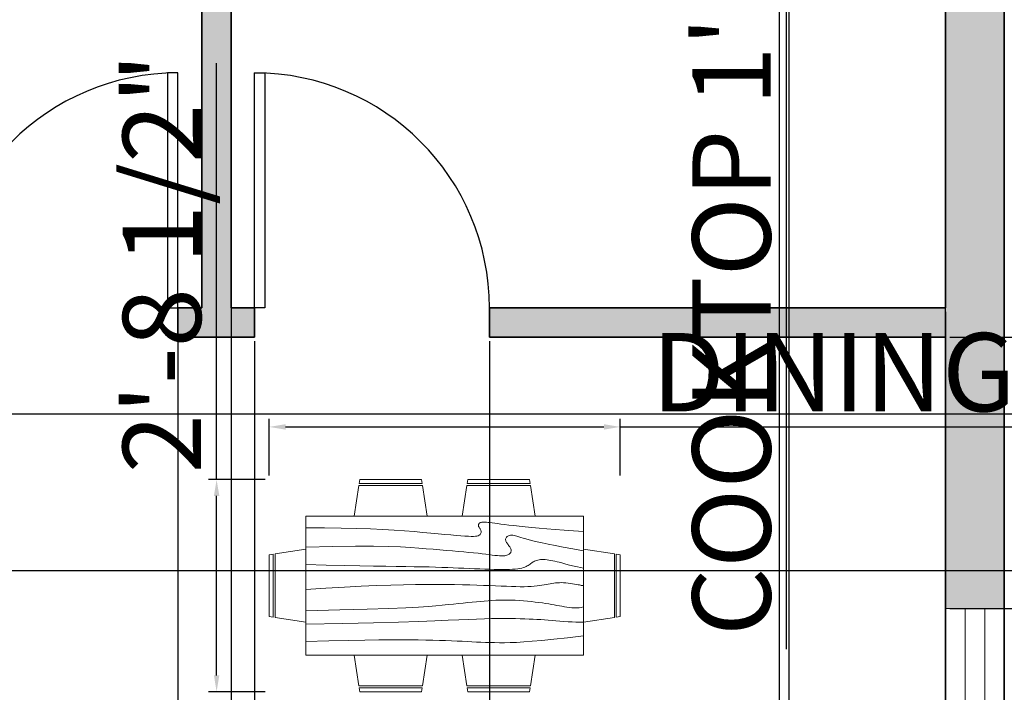
# Model space of a CAD drawing. Units: inches. Extents: x 1810 to 2254, y 313 to 1026.
# Tile 5 of 7: x 1988 to 2139, y 661 to 764. Entities that reach past the tile are written whole.
import ezdxf

# ---------------------------------------------------------------- set-up
doc = ezdxf.new("R2010")
doc.units = ezdxf.units.IN
for name, color, linetype, lineweight in [('A-ANNO-DIMS', 2, 'Continuous', 18), ('A-DOOR', 4, 'Continuous', 25), ('A-FLOR-CASE', 8, 'Continuous', 25), ('A-FURN', 8, 'Continuous', 18), ('A-GLAZ', 4, 'Continuous', 18), ('A-WALL', 7, 'Continuous', 35)]:
    doc.layers.add(name, color=color, linetype=linetype, lineweight=lineweight)
doc.layers.add('A-WALL-PATT', color=252, linetype='Continuous', lineweight=13, true_color=0x939598)
doc.styles.get("Standard").update_dxf_attribs({"font": 'arial.ttf'})
doc.dimstyles.new('ISO-25', dxfattribs={"dimtxt": 12, "dimasz": 2.5, "dimexe": 1.25, "dimexo": 0.625, "dimtad": 1, "dimdec": 1, "dimlunit": 4, "dimtxsty": 'Standard', "dimcen": 2.5, "dimadec": 0, "dimazin": 0, "dimtfac": 1, "dimtdec": 1, "dimtmove": 0, "dimatfit": 3, "dimfxl": 1, "dimarcsym": 0})

# ---------------------------------------------------------------- blocks, each defined once
blk = doc.blocks.new('A$C72FA0E17')
for p, q in [((0.5711, 1.3365), (0.5673, 1.3122)), ((0.9637, 1.3122), (0.5673, 1.3122)), ((0.5711, 1.3365), (0.9599, 1.3365)), ((0.9636, 1.3122), (0.9599, 1.3365)), ((1.2515, 1.3365), (1.2477, 1.3122)), ((1.6441, 1.3122), (1.2477, 1.3122)), ((1.2515, 1.3365), (1.6403, 1.3365)), ((1.644, 1.3122), (1.6403, 1.3365)), ((0.5654, 1.3001), (0.535, 1.1056)), ((0.5655, 1.3001), (0.9657, 1.3001)), ((0.9959, 1.1056), (0.9655, 1.3)), ((1.2458, 1.3001), (1.2154, 1.1056)), ((1.2459, 1.3001), (1.6461, 1.3001)), ((1.6763, 1.1056), (1.6459, 1.3)), ((1.9805, 1.1057), (0.2309, 1.1057)), ((0.2309, 1.1057), (0.2309, 0.2309)), ((1.3186, 1.0538), (1.3198, 1.0565)), ((1.3198, 1.0565), (1.3216, 1.0591)), ((1.3216, 1.0591), (1.324, 1.0614)), ((1.324, 1.0614), (1.3269, 1.0634)), ((1.3269, 1.0634), (1.3304, 1.0651)), ((1.3304, 1.0651), (1.3345, 1.0665)), ((1.3345, 1.0665), (1.3393, 1.0674)), ((1.3393, 1.0674), (1.345, 1.068)), ((1.345, 1.068), (1.3517, 1.0682)), ((1.3517, 1.0682), (1.3595, 1.068)), ((1.3595, 1.068), (1.3686, 1.0674)), ((1.3686, 1.0674), (1.3791, 1.0665)), ((1.3791, 1.0665), (1.3912, 1.0651)), ((1.3912, 1.0651), (1.405, 1.0634)), ((1.405, 1.0634), (1.4208, 1.0614)), ((1.4208, 1.0614), (1.4389, 1.059)), ((1.4389, 1.059), (1.4596, 1.0563)), ((1.4596, 1.0563), (1.4833, 1.0533)), ((1.9805, 0.2309), (1.9805, 1.1057)), ((0.2309, 1.0328), (0.348, 1.0322)), ((0.348, 1.0322), (0.4542, 1.0307)), ((0.4542, 1.0307), (0.5503, 1.0283)), ((0.5503, 1.0283), (0.6372, 1.0252)), ((0.6372, 1.0252), (0.716, 1.0215)), ((0.716, 1.0215), (0.7874, 1.0174)), ((0.7874, 1.0174), (0.8525, 1.013)), ((0.8525, 1.013), (0.9123, 1.0085)), ((0.9123, 1.0085), (0.9674, 1.0039)), ((0.9674, 1.0039), (1.0181, 0.9995)), ((1.0181, 0.9995), (1.0645, 0.9952)), ((1.0645, 0.9952), (1.1065, 0.9912)), ((1.3178, 1.0479), (1.3179, 1.0509)), ((1.3183, 1.0449), (1.3178, 1.0479)), ((1.3179, 1.0509), (1.3186, 1.0538)), ((1.3193, 1.0419), (1.3183, 1.0449)), ((1.3208, 1.0388), (1.3193, 1.0419)), ((1.3226, 1.0357), (1.3208, 1.0388)), ((1.3246, 1.0325), (1.3226, 1.0357)), ((1.3267, 1.0292), (1.3246, 1.0325)), ((1.3288, 1.0258), (1.3267, 1.0292)), ((1.3308, 1.0223), (1.3288, 1.0258)), ((1.3297, 0.9914), (1.3322, 0.9949)), ((1.3324, 1.0186), (1.3308, 1.0223)), ((1.3322, 0.9949), (1.3338, 0.9987)), ((1.3338, 1.0147), (1.3324, 1.0186)), ((1.3346, 1.0107), (1.3338, 1.0147)), ((1.3338, 0.9987), (1.3347, 1.0026)), ((1.335, 1.0067), (1.3346, 1.0107)), ((1.3347, 1.0026), (1.335, 1.0067)), ((1.4833, 1.0533), (1.5101, 1.0501)), ((1.5101, 1.0501), (1.5404, 1.0466)), ((1.5404, 1.0466), (1.5744, 1.0429)), ((1.5744, 1.0429), (1.6125, 1.039)), ((1.6125, 1.039), (1.6545, 1.0349)), ((1.6545, 1.0349), (1.7003, 1.0307)), ((1.7003, 1.0307), (1.7497, 1.0264)), ((1.7497, 1.0264), (1.8026, 1.022)), ((1.8026, 1.022), (1.8588, 1.0175)), ((1.8588, 1.0175), (1.9181, 1.013)), ((1.9181, 1.013), (1.9805, 1.0085)), ((1.1065, 0.9912), (1.1444, 0.9876)), ((1.1444, 0.9876), (1.1781, 0.9845)), ((1.1781, 0.9845), (1.2077, 0.982)), ((1.2077, 0.982), (1.2332, 0.9801)), ((1.2332, 0.9801), (1.2548, 0.979)), ((1.2548, 0.979), (1.2728, 0.9785)), ((1.2728, 0.9785), (1.2876, 0.9787)), ((1.2876, 0.9787), (1.2995, 0.9796)), ((1.2995, 0.9796), (1.309, 0.981)), ((1.309, 0.981), (1.3164, 0.9829)), ((1.3164, 0.9829), (1.322, 0.9854)), ((1.322, 0.9854), (1.3264, 0.9882)), ((1.3264, 0.9882), (1.3297, 0.9914)), ((1.4895, 0.9578), (1.4897, 0.962)), ((1.4901, 0.9535), (1.4895, 0.9578)), ((1.4897, 0.962), (1.4906, 0.9661)), ((1.4914, 0.9491), (1.4901, 0.9535)), ((1.4906, 0.9661), (1.4924, 0.97)), ((1.4933, 0.9446), (1.4914, 0.9491)), ((1.4924, 0.97), (1.4952, 0.9737)), ((1.4957, 0.9401), (1.4933, 0.9446)), ((1.4952, 0.9737), (1.4988, 0.9771)), ((1.4985, 0.9356), (1.4957, 0.9401)), ((1.5017, 0.931), (1.4985, 0.9356)), ((1.4988, 0.9771), (1.5032, 0.9801)), ((1.5051, 0.9264), (1.5017, 0.931)), ((1.5032, 0.9801), (1.5084, 0.9826)), ((1.5084, 0.9826), (1.5142, 0.9846)), ((1.5142, 0.9846), (1.5206, 0.9859)), ((1.5206, 0.9859), (1.5276, 0.9865)), ((1.5276, 0.9865), (1.535, 0.9862)), ((1.535, 0.9862), (1.5428, 0.985)), ((1.5428, 0.985), (1.5514, 0.9829)), ((1.5514, 0.9829), (1.561, 0.98)), ((1.561, 0.98), (1.572, 0.9764)), ((1.572, 0.9764), (1.5848, 0.9722)), ((1.5848, 0.9722), (1.5997, 0.9675)), ((1.5997, 0.9675), (1.6171, 0.9624)), ((1.6171, 0.9624), (1.6372, 0.9568)), ((1.6372, 0.9568), (1.6606, 0.9509)), ((1.6606, 0.9509), (1.6879, 0.9446)), ((1.6879, 0.9446), (1.7199, 0.9376)), ((1.7199, 0.9376), (1.7576, 0.9299)), ((0.0364, 0.8683), (0.2309, 0.8987)), ((0.2309, 0.9113), (0.4015, 0.9147)), ((0.4015, 0.9147), (0.5426, 0.9162)), ((0.5426, 0.9162), (0.6579, 0.9161)), ((0.6579, 0.9161), (0.7517, 0.9145)), ((0.7517, 0.9145), (0.8277, 0.912)), ((0.8277, 0.912), (0.8899, 0.9087)), ((0.8899, 0.9087), (0.9425, 0.905)), ((0.9425, 0.905), (0.9892, 0.9011)), ((0.9892, 0.9011), (1.0335, 0.8974)), ((1.0335, 0.8974), (1.0759, 0.8939)), ((1.0759, 0.8939), (1.1164, 0.8905)), ((1.1164, 0.8905), (1.1549, 0.8872)), ((1.1549, 0.8872), (1.1913, 0.884)), ((1.1913, 0.884), (1.2257, 0.8809)), ((1.2257, 0.8809), (1.2579, 0.8778)), ((1.2579, 0.8778), (1.2879, 0.8748)), ((1.2879, 0.8748), (1.3156, 0.8718)), ((1.3156, 0.8718), (1.3412, 0.8688)), ((1.3412, 0.8688), (1.3645, 0.866)), ((1.5087, 0.9219), (1.5051, 0.9264)), ((1.5122, 0.9173), (1.5087, 0.9219)), ((1.5155, 0.9128), (1.5122, 0.9173)), ((1.5127, 0.8667), (1.5162, 0.8699)), ((1.5184, 0.9082), (1.5155, 0.9128)), ((1.5162, 0.8699), (1.5191, 0.8735)), ((1.5209, 0.9037), (1.5184, 0.9082)), ((1.5191, 0.8735), (1.5214, 0.8773)), ((1.5228, 0.8991), (1.5209, 0.9037)), ((1.5214, 0.8773), (1.5231, 0.8814)), ((1.5239, 0.8946), (1.5228, 0.8991)), ((1.5231, 0.8814), (1.524, 0.8856)), ((1.5244, 0.8901), (1.5239, 0.8946)), ((1.524, 0.8856), (1.5244, 0.8901)), ((1.7576, 0.9299), (1.8016, 0.9211)), ((1.8016, 0.9211), (1.8529, 0.9111)), ((1.8529, 0.9111), (1.9123, 0.8998)), ((1.9123, 0.8998), (1.9805, 0.887)), ((2.1749, 0.8683), (1.9804, 0.8987)), ((0, 0.8627), (0.0243, 0.8664)), ((0, 0.8627), (0, 0.4739)), ((0.0243, 0.47), (0.0243, 0.8664)), ((0.0365, 0.8682), (0.0365, 0.468)), ((1.3645, 0.866), (1.3859, 0.8634)), ((1.3859, 0.8634), (1.4052, 0.8611)), ((1.4052, 0.8611), (1.4226, 0.8591)), ((1.4226, 0.8591), (1.4381, 0.8576)), ((1.4381, 0.8576), (1.4519, 0.8566)), ((1.4519, 0.8566), (1.464, 0.8561)), ((1.464, 0.8561), (1.4745, 0.8562)), ((1.4745, 0.8562), (1.4836, 0.8568)), ((1.4836, 0.8568), (1.4914, 0.8578)), ((1.4914, 0.8578), (1.4981, 0.8594)), ((1.4981, 0.8594), (1.5038, 0.8614)), ((1.5038, 0.8614), (1.5086, 0.8639)), ((1.5086, 0.8639), (1.5127, 0.8667)), ((1.6439, 0.8041), (1.6492, 0.8081)), ((1.6492, 0.8081), (1.6544, 0.812)), ((1.6544, 0.812), (1.6598, 0.8157)), ((1.6598, 0.8157), (1.6655, 0.8192)), ((1.6655, 0.8192), (1.6715, 0.8223)), ((1.6715, 0.8223), (1.678, 0.8252)), ((1.678, 0.8252), (1.6849, 0.8276)), ((1.6849, 0.8276), (1.6923, 0.8297)), ((1.6923, 0.8297), (1.7004, 0.8312)), ((1.7004, 0.8312), (1.7091, 0.8323)), ((1.7091, 0.8323), (1.7186, 0.8328)), ((1.7186, 0.8328), (1.7288, 0.8327)), ((1.7288, 0.8327), (1.7395, 0.8321)), ((1.7395, 0.8321), (1.7509, 0.831)), ((1.7509, 0.831), (1.7627, 0.8294)), ((1.7627, 0.8294), (1.7749, 0.8274)), ((1.7749, 0.8274), (1.7874, 0.825)), ((1.7874, 0.825), (1.8002, 0.8221)), ((1.8002, 0.8221), (1.8134, 0.8189)), ((1.8134, 0.8189), (1.8275, 0.8152)), ((1.8275, 0.8152), (1.8435, 0.8109)), ((1.8435, 0.8109), (1.8622, 0.8059)), ((2.1749, 0.8682), (2.1749, 0.468)), ((2.2113, 0.8627), (2.187, 0.8664)), ((2.187, 0.47), (2.187, 0.8664)), ((2.2113, 0.8627), (2.2113, 0.4739)), ((0.2309, 0.8019), (0.3593, 0.7979)), ((0.3593, 0.7979), (0.4722, 0.7948)), ((0.4722, 0.7948), (0.5712, 0.7926)), ((0.5712, 0.7926), (0.6579, 0.791)), ((0.6579, 0.791), (0.7338, 0.7899)), ((0.7338, 0.7899), (0.8007, 0.7891)), ((0.8007, 0.7891), (0.8599, 0.7884)), ((0.8599, 0.7884), (0.9133, 0.7877)), ((0.9133, 0.7877), (0.9621, 0.7869)), ((0.9621, 0.7869), (1.007, 0.7859)), ((1.007, 0.7859), (1.0487, 0.7847)), ((1.0487, 0.7847), (1.0877, 0.7834)), ((1.0877, 0.7834), (1.1245, 0.782)), ((1.1245, 0.782), (1.1596, 0.7806)), ((1.1596, 0.7806), (1.1936, 0.7791)), ((1.1936, 0.7791), (1.2272, 0.7776)), ((1.2272, 0.7776), (1.2605, 0.7761)), ((1.2605, 0.7761), (1.2936, 0.7746)), ((1.2936, 0.7746), (1.3261, 0.7733)), ((1.3261, 0.7733), (1.3578, 0.772)), ((1.3578, 0.772), (1.3883, 0.771)), ((1.3883, 0.771), (1.4174, 0.7702)), ((1.4174, 0.7702), (1.4448, 0.7697)), ((1.4448, 0.7697), (1.4702, 0.7695)), ((1.4702, 0.7695), (1.4933, 0.7697)), ((1.4933, 0.7697), (1.5144, 0.7703)), ((1.5144, 0.7703), (1.5333, 0.7712)), ((1.5333, 0.7712), (1.5504, 0.7725)), ((1.5504, 0.7725), (1.5656, 0.7742)), ((1.5656, 0.7742), (1.5792, 0.7763)), ((1.5792, 0.7763), (1.5912, 0.7788)), ((1.5912, 0.7788), (1.6018, 0.7816)), ((1.6018, 0.7816), (1.611, 0.7849)), ((1.611, 0.7849), (1.6191, 0.7884)), ((1.6191, 0.7884), (1.6263, 0.7922)), ((1.6263, 0.7922), (1.6327, 0.7961)), ((1.6327, 0.7961), (1.6385, 0.8001)), ((1.6385, 0.8001), (1.6439, 0.8041)), ((1.8622, 0.8059), (1.8844, 0.8002)), ((1.8844, 0.8002), (1.911, 0.7937)), ((1.911, 0.7937), (1.9427, 0.7862)), ((1.9427, 0.7862), (1.9805, 0.7776)), ((1.7814, 0.6825), (1.7931, 0.6841)), ((1.7931, 0.6841), (1.8048, 0.6855)), ((1.8048, 0.6855), (1.8167, 0.6864)), ((1.8167, 0.6864), (1.8289, 0.6869)), ((1.8289, 0.6869), (1.8416, 0.687)), ((1.8416, 0.687), (1.8549, 0.6865)), ((1.8549, 0.6865), (1.8689, 0.6855)), ((1.8689, 0.6855), (1.8832, 0.684)), ((1.8832, 0.684), (1.8976, 0.6822)), ((0.2309, 0.644), (0.3574, 0.6522)), ((0.3574, 0.6522), (0.4734, 0.659)), ((0.4734, 0.659), (0.5795, 0.6643)), ((0.5795, 0.6643), (0.6766, 0.6684)), ((0.6766, 0.6684), (0.7654, 0.6714)), ((0.7654, 0.6714), (0.8468, 0.6734)), ((0.8468, 0.6734), (0.9215, 0.6747)), ((0.9215, 0.6747), (0.9902, 0.6753)), ((0.9902, 0.6753), (1.0538, 0.6755)), ((1.0538, 0.6755), (1.1126, 0.6752)), ((1.1126, 0.6752), (1.1672, 0.6746)), ((1.1672, 0.6746), (1.2178, 0.6737)), ((1.2178, 0.6737), (1.2649, 0.6725)), ((1.2649, 0.6725), (1.3089, 0.6712)), ((1.3089, 0.6712), (1.3502, 0.6698)), ((1.3502, 0.6698), (1.3892, 0.6683)), ((1.3892, 0.6683), (1.4262, 0.6667)), ((1.4262, 0.6667), (1.4613, 0.6653)), ((1.4613, 0.6653), (1.4944, 0.664)), ((1.4944, 0.664), (1.5256, 0.6629)), ((1.5256, 0.6629), (1.5548, 0.6621)), ((1.5548, 0.6621), (1.5819, 0.6617)), ((1.5819, 0.6617), (1.6071, 0.6617)), ((1.6071, 0.6617), (1.6301, 0.6622)), ((1.6301, 0.6622), (1.6511, 0.6632)), ((1.6511, 0.6632), (1.6703, 0.6647)), ((1.6703, 0.6647), (1.6878, 0.6666)), ((1.6878, 0.6666), (1.7038, 0.6688)), ((1.7038, 0.6688), (1.7186, 0.6711)), ((1.7186, 0.6711), (1.7324, 0.6736)), ((1.7324, 0.6736), (1.7453, 0.676)), ((1.7453, 0.676), (1.7577, 0.6784)), ((1.7577, 0.6784), (1.7697, 0.6806)), ((1.7697, 0.6806), (1.7814, 0.6825)), ((1.8976, 0.6822), (1.9115, 0.6801)), ((1.9115, 0.6801), (1.9246, 0.678)), ((1.9246, 0.678), (1.9365, 0.6759)), ((1.9365, 0.6759), (1.9468, 0.674)), ((1.9468, 0.674), (1.9551, 0.6723)), ((1.9551, 0.6723), (1.9613, 0.671)), ((1.9613, 0.671), (1.9655, 0.67)), ((1.9655, 0.67), (1.9684, 0.6692)), ((1.9684, 0.6692), (1.9705, 0.6688)), ((1.9705, 0.6688), (1.9722, 0.6685)), ((1.9722, 0.6685), (1.9741, 0.6683)), ((1.9741, 0.6683), (1.9767, 0.6683)), ((1.9767, 0.6683), (1.9805, 0.6683)), ((1.223, 0.5584), (1.2516, 0.5613)), ((1.2516, 0.5613), (1.2788, 0.5641)), ((1.2788, 0.5641), (1.305, 0.5667)), ((1.305, 0.5667), (1.3304, 0.569)), ((1.3304, 0.569), (1.3552, 0.5712)), ((1.3552, 0.5712), (1.3796, 0.5731)), ((1.3796, 0.5731), (1.4037, 0.5748)), ((1.4037, 0.5748), (1.4276, 0.5761)), ((1.4276, 0.5761), (1.4516, 0.5771)), ((1.4516, 0.5771), (1.4757, 0.5776)), ((1.4757, 0.5776), (1.5, 0.5776)), ((1.5, 0.5776), (1.5248, 0.5771)), ((1.5248, 0.5771), (1.5501, 0.5761)), ((1.5501, 0.5761), (1.5757, 0.5746)), ((1.5757, 0.5746), (1.6014, 0.5726)), ((1.6014, 0.5726), (1.6268, 0.5703)), ((1.6268, 0.5703), (1.6518, 0.5677)), ((1.6518, 0.5677), (1.676, 0.5649)), ((1.676, 0.5649), (1.6993, 0.5619)), ((1.6993, 0.5619), (1.7213, 0.5589)), ((1.7213, 0.5589), (1.7418, 0.5559)), ((0.2309, 0.5103), (0.4451, 0.5149)), ((0.4451, 0.5149), (0.6176, 0.5194)), ((0.6176, 0.5194), (0.7541, 0.5239)), ((0.7541, 0.5239), (0.86, 0.5283)), ((0.86, 0.5283), (0.941, 0.5326)), ((0.941, 0.5326), (1.0027, 0.5368)), ((1.0027, 0.5368), (1.0507, 0.5408)), ((1.0507, 0.5408), (1.0905, 0.5447)), ((1.0905, 0.5447), (1.1268, 0.5484)), ((1.1268, 0.5484), (1.1608, 0.5519)), ((1.1608, 0.5519), (1.1928, 0.5553)), ((1.1928, 0.5553), (1.223, 0.5584)), ((1.7418, 0.5559), (1.761, 0.5528)), ((1.761, 0.5528), (1.7791, 0.5498)), ((1.7791, 0.5498), (1.7963, 0.5469)), ((1.7963, 0.5469), (1.8128, 0.544)), ((1.8128, 0.544), (1.8288, 0.5411)), ((1.8288, 0.5411), (1.8444, 0.5383)), ((1.8444, 0.5383), (1.86, 0.5356)), ((1.86, 0.5356), (1.8756, 0.533)), ((1.8756, 0.533), (1.8912, 0.5308)), ((1.8912, 0.5308), (1.9067, 0.529)), ((1.9067, 0.529), (1.9221, 0.5279)), ((1.9221, 0.5279), (1.9373, 0.5277)), ((1.9373, 0.5277), (1.9521, 0.5286)), ((1.9521, 0.5286), (1.9665, 0.5309)), ((1.9665, 0.5309), (1.9805, 0.5346)), ((0.0243, 0.4701), (0, 0.4739)), ((0.2309, 0.4378), (0.0365, 0.4682)), ((0.6569, 0.4343), (0.8144, 0.4386)), ((0.8144, 0.4386), (0.9419, 0.4427)), ((0.9419, 0.4427), (1.0444, 0.4465)), ((1.0444, 0.4465), (1.127, 0.45)), ((1.127, 0.45), (1.195, 0.4531)), ((1.195, 0.4531), (1.2535, 0.4556)), ((1.2535, 0.4556), (1.3068, 0.4576)), ((1.3068, 0.4576), (1.356, 0.4591)), ((1.356, 0.4591), (1.4014, 0.4601)), ((1.4014, 0.4601), (1.4433, 0.4607)), ((1.4433, 0.4607), (1.482, 0.4609)), ((1.482, 0.4609), (1.5177, 0.4608)), ((1.5177, 0.4608), (1.5508, 0.4603)), ((1.5508, 0.4603), (1.5815, 0.4597)), ((1.5815, 0.4597), (1.6102, 0.4588)), ((1.6102, 0.4588), (1.6371, 0.4578)), ((1.6371, 0.4578), (1.6626, 0.4566)), ((1.6626, 0.4566), (1.6871, 0.4552)), ((1.6871, 0.4552), (1.7109, 0.4538)), ((1.7109, 0.4538), (1.7344, 0.4521)), ((1.7344, 0.4521), (1.758, 0.4504)), ((1.758, 0.4504), (1.782, 0.4485)), ((1.782, 0.4485), (1.8066, 0.4466)), ((1.8066, 0.4466), (1.8318, 0.4447)), ((1.8318, 0.4447), (1.8572, 0.4428)), ((1.8572, 0.4428), (1.8827, 0.4411)), ((1.8827, 0.4411), (1.908, 0.4396)), ((1.908, 0.4396), (1.9329, 0.4384)), ((1.9329, 0.4384), (1.9571, 0.4377)), ((1.9571, 0.4377), (1.9805, 0.4374)), ((1.9804, 0.4378), (2.1748, 0.4682)), ((2.187, 0.4701), (2.2113, 0.4739)), ((0.2309, 0.4253), (0.4641, 0.4298)), ((0.4641, 0.4298), (0.6569, 0.4343)), ((0.2309, 0.3159), (0.3745, 0.3199)), ((0.3745, 0.3199), (0.4973, 0.3229)), ((0.4973, 0.3229), (0.6019, 0.325)), ((0.6019, 0.325), (0.6907, 0.3263)), ((0.6907, 0.3263), (0.7662, 0.3269)), ((0.7662, 0.3269), (0.831, 0.327)), ((0.831, 0.327), (0.8876, 0.3267)), ((0.8876, 0.3267), (0.9386, 0.326)), ((0.9386, 0.326), (0.986, 0.3252)), ((0.986, 0.3252), (1.0306, 0.3242)), ((1.0306, 0.3242), (1.0723, 0.323)), ((1.0723, 0.323), (1.1116, 0.3217)), ((1.1116, 0.3217), (1.1485, 0.3203)), ((1.1485, 0.3203), (1.1833, 0.3189)), ((1.1833, 0.3189), (1.2162, 0.3174)), ((1.2162, 0.3174), (1.2474, 0.3159)), ((1.2474, 0.3159), (1.2771, 0.3144)), ((1.2771, 0.3144), (1.3058, 0.3129)), ((1.3058, 0.3129), (1.3339, 0.3116)), ((1.3339, 0.3116), (1.3619, 0.3105)), ((1.3619, 0.3105), (1.3904, 0.3095)), ((1.5186, 0.3095), (1.558, 0.3109)), ((1.558, 0.3109), (1.6033, 0.3134)), ((1.6033, 0.3134), (1.6563, 0.3173)), ((1.6563, 0.3173), (1.7188, 0.3228)), ((1.7188, 0.3228), (1.7924, 0.3303)), ((1.7924, 0.3303), (1.8791, 0.3401)), ((1.8791, 0.3401), (1.9805, 0.3524)), ((1.3904, 0.3095), (1.4198, 0.3089)), ((1.4198, 0.3089), (1.4506, 0.3087)), ((1.4506, 0.3087), (1.4833, 0.3088)), ((1.4833, 0.3088), (1.5186, 0.3095)), ((0.2309, 0.2309), (1.9805, 0.2309)), ((0.5654, 0.0364), (0.535, 0.2309)), ((0.9959, 0.2309), (0.9655, 0.0365)), ((1.2458, 0.0364), (1.2154, 0.2309)), ((1.6763, 0.2309), (1.6459, 0.0365)), ((0.5655, 0.0365), (0.9657, 0.0365)), ((0.5711, 0), (0.5673, 0.0243)), ((0.9637, 0.0243), (0.5673, 0.0243)), ((0.5711, 0), (0.9599, 0)), ((0.9636, 0.0243), (0.9599, 0)), ((1.2459, 0.0365), (1.6461, 0.0365)), ((1.2515, 0), (1.2477, 0.0243)), ((1.6441, 0.0243), (1.2477, 0.0243)), ((1.2515, 0), (1.6403, 0)), ((1.644, 0.0243), (1.6403, 0))]:
    blk.add_line(p, q)
blk = doc.blocks.new('*U18')
for p, q in [((0, 0), (0, -4)), ((40, 0), (40, -4))]:
    blk.add_line(p, q)
blk.add_lwpolyline([(0, 0), (0, 40), (1.75, 40), (1.75, 0)], close=True)
blk.add_arc((0, 0), 40, 0, 90)
blk = doc.blocks.new('*U17')
for p, q in [((0, 0), (0, -4)), ((-40, 0), (-40, -4))]:
    blk.add_line(p, q)
blk.add_lwpolyline([(0, 0), (0, 40), (-1.75, 40), (-1.75, 0)], close=True)
blk.add_arc((0, 0), 40, 90, 180)
blk = doc.blocks.new('*D23')
at = {"layer": 'A-ANNO-DIMS', "color": 0, "lineweight": -2, "transparency": 16777216}
for p, q in [((2130.99, 851.61), (2253.63, 851.61)), ((2252.38, 849.11), (2252.38, 437.11)), ((2130.99, 434.61), (2253.63, 434.61))]:
    blk.add_line(p, q, dxfattribs=at)
at = {"layer": 'A-ANNO-DIMS', "color": 0, "transparency": 16777216}
for points in [[(2251.96, 849.11), (2252.8, 849.11), (2252.38, 851.61)], [(2251.96, 437.11), (2252.8, 437.11), (2252.38, 434.61)]]:
    blk.add_solid(points, dxfattribs=at)
at = {"layer": 'Defpoints', "color": 0, "transparency": 16777216}
for p in [(2130.36, 851.61), (2130.36, 434.61), (2252.38, 434.61)]:
    blk.add_point(p, dxfattribs=at)
at = {"layer": 'A-ANNO-DIMS', "color": 0, "transparency": 16777216, "insert": (2245.62, 643.11), "char_height": 12, "attachment_point": 5, "rotation": 90}
blk.add_mtext('34\'-9"', dxfattribs=at)
blk = doc.blocks.new('WIN-36IN-WALL9')
for p, q in [((0, 9), (0, 0)), ((36, 9), (36, 0)), ((0, 6), (36, 6)), ((0, 3), (36, 3))]:
    blk.add_line(p, q)
blk = doc.blocks.new('*D42')
at = {"layer": 'A-ANNO-DIMS', "color": 0, "lineweight": -2, "transparency": 16777216}
for p, q in [((2108.19, 810.48), (2104.68, 810.48)), ((2105.93, 807.98), (2105.93, 793.78)), ((2108.19, 791.28), (2104.68, 791.28)), ((2105.93, 791.28), (2105.93, 667.28))]:
    blk.add_line(p, q, dxfattribs=at)
at = {"layer": 'A-ANNO-DIMS', "color": 0, "transparency": 16777216}
for points in [[(2105.52, 807.98), (2106.35, 807.98), (2105.93, 810.48)], [(2105.52, 793.78), (2106.35, 793.78), (2105.93, 791.28)]]:
    blk.add_solid(points, dxfattribs=at)
at = {"layer": 'Defpoints', "color": 0, "transparency": 16777216}
for p in [(2108.81, 810.48), (2105.93, 791.28), (2108.81, 791.28)]:
    blk.add_point(p, dxfattribs=at)
at = {"layer": 'A-ANNO-DIMS', "color": 0, "transparency": 16777216, "insert": (2099.1, 728.03), "char_height": 12, "attachment_point": 5, "rotation": 90}
blk.add_mtext('COOKTOP 1\'-7"', dxfattribs=at)
blk = doc.blocks.new('*D46')
at = {"layer": 'A-ANNO-DIMS', "color": 0, "lineweight": -2, "transparency": 16777216}
for p, q in [((2026.69, 693.91), (2026.69, 702.6)), ((2080.48, 693.91), (2080.48, 702.6)), ((2029.19, 701.35), (2077.98, 701.35)), ((2080.48, 701.35), (2216.12, 701.35))]:
    blk.add_line(p, q, dxfattribs=at)
at = {"layer": 'A-ANNO-DIMS', "color": 0, "transparency": 16777216}
for points in [[(2029.19, 701.77), (2029.19, 700.93), (2026.69, 701.35)], [(2077.98, 701.77), (2077.98, 700.93), (2080.48, 701.35)]]:
    blk.add_solid(points, dxfattribs=at)
at = {"layer": 'Defpoints', "color": 0, "transparency": 16777216}
for p in [(2080.48, 701.35), (2026.69, 693.28), (2080.48, 693.28)]:
    blk.add_point(p, dxfattribs=at)
at = {"layer": 'A-ANNO-DIMS', "color": 0, "transparency": 16777216, "insert": (2149.55, 708.18), "char_height": 12, "attachment_point": 5}
blk.add_mtext('DINING SET 4\'-6"', dxfattribs=at)
blk = doc.blocks.new('*D47')
at = {"layer": 'A-ANNO-DIMS', "color": 0, "lineweight": -2, "transparency": 16777216}
for p, q in [((2018.62, 693.28), (2018.62, 757.1)), ((2026.07, 693.28), (2017.37, 693.28)), ((2018.62, 663.27), (2018.62, 690.78)), ((2026.07, 660.77), (2017.37, 660.77))]:
    blk.add_line(p, q, dxfattribs=at)
at = {"layer": 'A-ANNO-DIMS', "color": 0, "transparency": 16777216}
for points in [[(2018.21, 690.78), (2019.04, 690.78), (2018.62, 693.28)], [(2018.21, 663.27), (2019.04, 663.27), (2018.62, 660.77)]]:
    blk.add_solid(points, dxfattribs=at)
at = {"layer": 'Defpoints', "color": 0, "transparency": 16777216}
for p in [(2018.62, 693.28), (2026.69, 693.28), (2026.69, 660.77)]:
    blk.add_point(p, dxfattribs=at)
at = {"layer": 'A-ANNO-DIMS', "color": 0, "transparency": 16777216, "insert": (2011.79, 726.44), "char_height": 12, "attachment_point": 5, "rotation": 90}
blk.add_mtext('2\'-8 1/2"', dxfattribs=at)
blk = doc.blocks.new('*D54')
at = {"layer": 'A-ANNO-DIMS', "color": 0, "lineweight": -2, "transparency": 16777216}
for p, q in [((2130.99, 715.11), (2162.01, 715.11)), ((2160.76, 712.61), (2160.76, 676.02)), ((2130.99, 673.52), (2162.01, 673.52)), ((2160.76, 673.52), (2160.76, 609.92))]:
    blk.add_line(p, q, dxfattribs=at)
at = {"layer": 'A-ANNO-DIMS', "color": 0, "transparency": 16777216}
for points in [[(2160.35, 712.61), (2161.18, 712.61), (2160.76, 715.11)], [(2160.35, 676.02), (2161.18, 676.02), (2160.76, 673.52)]]:
    blk.add_solid(points, dxfattribs=at)
at = {"layer": 'Defpoints', "color": 0, "transparency": 16777216}
for p in [(2130.36, 715.11), (2130.36, 673.52), (2160.76, 673.52)]:
    blk.add_point(p, dxfattribs=at)
at = {"layer": 'A-ANNO-DIMS', "color": 0, "transparency": 16777216, "insert": (2153.93, 640.47), "char_height": 12, "attachment_point": 5, "rotation": 90}
blk.add_mtext('3\'-5 1/2"', dxfattribs=at)
blk = doc.blocks.new('*D57')
at = {"layer": 'A-ANNO-DIMS', "color": 0, "lineweight": -2, "transparency": 16777216}
for p, q in [((2104.86, 718.99), (2104.86, 323.71)), ((2130.36, 718.99), (2130.36, 323.71)), ((2107.36, 324.96), (2127.86, 324.96)), ((2130.36, 324.96), (2194.18, 324.96))]:
    blk.add_line(p, q, dxfattribs=at)
at = {"layer": 'A-ANNO-DIMS', "color": 0, "transparency": 16777216}
for points in [[(2107.36, 325.38), (2107.36, 324.55), (2104.86, 324.96)], [(2127.86, 325.38), (2127.86, 324.55), (2130.36, 324.96)]]:
    blk.add_solid(points, dxfattribs=at)
at = {"layer": 'Defpoints', "color": 0, "transparency": 16777216}
for p in [(2104.86, 719.61), (2130.36, 719.61), (2130.36, 324.96)]:
    blk.add_point(p, dxfattribs=at)
at = {"layer": 'A-ANNO-DIMS', "color": 0, "transparency": 16777216, "insert": (2163.52, 331.79), "char_height": 12, "attachment_point": 5}
blk.add_mtext('2\'-1 1/2"', dxfattribs=at)
blk = doc.blocks.new('*D59')
at = {"layer": 'A-ANNO-DIMS', "color": 0, "lineweight": -2, "transparency": 16777216}
for p, q in [((2024.44, 714.49), (2024.44, 323.71)), ((2060.44, 714.49), (2060.44, 323.71)), ((2026.94, 324.96), (2057.94, 324.96))]:
    blk.add_line(p, q, dxfattribs=at)
at = {"layer": 'A-ANNO-DIMS', "color": 0, "transparency": 16777216}
for points in [[(2026.94, 325.38), (2026.94, 324.55), (2024.44, 324.96)], [(2057.94, 325.38), (2057.94, 324.55), (2060.44, 324.96)]]:
    blk.add_solid(points, dxfattribs=at)
at = {"layer": 'Defpoints', "color": 0, "transparency": 16777216}
for p in [(2024.44, 715.11), (2060.44, 715.11), (2060.44, 324.96)]:
    blk.add_point(p, dxfattribs=at)
at = {"layer": 'A-ANNO-DIMS', "color": 0, "transparency": 16777216, "insert": (2042.44, 331.72), "char_height": 12, "attachment_point": 5}
blk.add_mtext('3\'-0"', dxfattribs=at)
blk = doc.blocks.new('*D61')
at = {"layer": 'A-ANNO-DIMS', "color": 0, "lineweight": -2, "transparency": 16777216}
for p, q in [((2106.36, 559.74), (2106.36, 892.26)), ((2130.36, 559.74), (2130.36, 892.26)), ((2108.86, 891.01), (2127.86, 891.01)), ((2130.36, 891.01), (2166.22, 891.01))]:
    blk.add_line(p, q, dxfattribs=at)
at = {"layer": 'A-ANNO-DIMS', "color": 0, "transparency": 16777216}
for points in [[(2108.86, 891.43), (2108.86, 890.6), (2106.36, 891.01)], [(2127.86, 891.43), (2127.86, 890.6), (2130.36, 891.01)]]:
    blk.add_solid(points, dxfattribs=at)
at = {"layer": 'Defpoints', "color": 0, "transparency": 16777216}
for p in [(2130.36, 891.01), (2106.36, 559.11), (2130.36, 559.11)]:
    blk.add_point(p, dxfattribs=at)
at = {"layer": 'A-ANNO-DIMS', "color": 0, "transparency": 16777216, "insert": (2149.54, 897.76), "char_height": 12, "attachment_point": 5}
blk.add_mtext('2\'-0"', dxfattribs=at)
blk = doc.blocks.new('*D62')
at = {"layer": 'A-ANNO-DIMS', "color": 0, "lineweight": -2, "transparency": 16777216}
for p, q in [((2169.76, 703.36), (2169.76, 739.21)), ((1973.49, 703.36), (2171.01, 703.36)), ((2169.76, 681.86), (2169.76, 700.86)), ((1973.49, 679.36), (2171.01, 679.36))]:
    blk.add_line(p, q, dxfattribs=at)
at = {"layer": 'A-ANNO-DIMS', "color": 0, "transparency": 16777216}
for points in [[(2169.35, 700.86), (2170.18, 700.86), (2169.76, 703.36)], [(2169.35, 681.86), (2170.18, 681.86), (2169.76, 679.36)]]:
    blk.add_solid(points, dxfattribs=at)
at = {"layer": 'Defpoints', "color": 0, "transparency": 16777216}
for p in [(1972.86, 703.36), (2169.76, 703.36), (1972.86, 679.36)]:
    blk.add_point(p, dxfattribs=at)
at = {"layer": 'A-ANNO-DIMS', "color": 0, "transparency": 16777216, "insert": (2163.01, 722.54), "char_height": 12, "attachment_point": 5, "rotation": 90}
blk.add_mtext('2\'-0"', dxfattribs=at)
blk = doc.blocks.new('*D63')
at = {"layer": 'A-ANNO-DIMS', "color": 0, "lineweight": -2, "transparency": 16777216}
for p, q in [((2169.76, 679.36), (2169.76, 715.21)), ((1973.49, 679.36), (2171.01, 679.36)), ((2169.76, 649.92), (2169.76, 676.86)), ((1973.49, 647.42), (2171.01, 647.42))]:
    blk.add_line(p, q, dxfattribs=at)
at = {"layer": 'A-ANNO-DIMS', "color": 0, "transparency": 16777216}
for points in [[(2169.35, 676.86), (2170.18, 676.86), (2169.76, 679.36)], [(2169.35, 649.92), (2170.18, 649.92), (2169.76, 647.42)]]:
    blk.add_solid(points, dxfattribs=at)
at = {"layer": 'Defpoints', "color": 0, "transparency": 16777216}
for p in [(1972.86, 679.36), (2169.76, 679.36), (1972.86, 647.42)]:
    blk.add_point(p, dxfattribs=at)
at = {"layer": 'A-ANNO-DIMS', "color": 0, "transparency": 16777216, "insert": (2163.01, 698.54), "char_height": 12, "attachment_point": 5, "rotation": 90}
blk.add_mtext('2\'-8"', dxfattribs=at)
blk = doc.blocks.new('*D65')
at = {"layer": 'A-ANNO-DIMS', "color": 0, "lineweight": -2, "transparency": 16777216}
for p, q in [((1968.36, 679.98), (1968.36, 892.26)), ((1972.86, 679.98), (1972.86, 892.26)), ((1965.86, 891.01), (1963.36, 891.01)), ((1968.36, 891.01), (1972.86, 891.01)), ((1975.36, 891.01), (2038.97, 891.01))]:
    blk.add_line(p, q, dxfattribs=at)
at = {"layer": 'A-ANNO-DIMS', "color": 0, "transparency": 16777216}
for points in [[(1965.86, 891.43), (1965.86, 890.6), (1968.36, 891.01)], [(1975.36, 891.43), (1975.36, 890.6), (1972.86, 891.01)]]:
    blk.add_solid(points, dxfattribs=at)
at = {"layer": 'Defpoints', "color": 0, "transparency": 16777216}
for p in [(1972.86, 891.01), (1968.36, 679.36), (1972.86, 679.36)]:
    blk.add_point(p, dxfattribs=at)
at = {"layer": 'A-ANNO-DIMS', "color": 0, "transparency": 16777216, "insert": (2008.42, 897.84), "char_height": 12, "attachment_point": 5}
blk.add_mtext('0\'-4 1/2"', dxfattribs=at)
blk = doc.blocks.new('*D67')
at = {"layer": 'A-ANNO-DIMS', "color": 0, "lineweight": -2, "transparency": 16777216}
for p, q in [((1976.68, 714.49), (1976.68, 323.71)), ((2012.68, 714.49), (2012.68, 323.71)), ((1979.18, 324.96), (2010.18, 324.96))]:
    blk.add_line(p, q, dxfattribs=at)
at = {"layer": 'A-ANNO-DIMS', "color": 0, "transparency": 16777216}
for points in [[(1979.18, 325.38), (1979.18, 324.55), (1976.68, 324.96)], [(2010.18, 325.38), (2010.18, 324.55), (2012.68, 324.96)]]:
    blk.add_solid(points, dxfattribs=at)
at = {"layer": 'Defpoints', "color": 0, "transparency": 16777216}
for p in [(1976.68, 715.11), (2012.68, 715.11), (2012.68, 324.96)]:
    blk.add_point(p, dxfattribs=at)
at = {"layer": 'A-ANNO-DIMS', "color": 0, "transparency": 16777216, "insert": (1994.68, 331.72), "char_height": 12, "attachment_point": 5}
blk.add_mtext('3\'-0"', dxfattribs=at)
blk = doc.blocks.new('*D68')
at = {"layer": 'A-ANNO-DIMS', "color": 0, "lineweight": -2, "transparency": 16777216}
for p, q in [((2020.86, 826.99), (2020.86, 323.71)), ((2104.86, 826.99), (2104.86, 323.71)), ((2023.36, 324.96), (2102.36, 324.96))]:
    blk.add_line(p, q, dxfattribs=at)
at = {"layer": 'A-ANNO-DIMS', "color": 0, "transparency": 16777216}
for points in [[(2023.36, 325.38), (2023.36, 324.55), (2020.86, 324.96)], [(2102.36, 325.38), (2102.36, 324.55), (2104.86, 324.96)]]:
    blk.add_solid(points, dxfattribs=at)
at = {"layer": 'Defpoints', "color": 0, "transparency": 16777216}
for p in [(2020.86, 827.61), (2104.86, 827.61), (2104.86, 324.96)]:
    blk.add_point(p, dxfattribs=at)
at = {"layer": 'A-ANNO-DIMS', "color": 0, "transparency": 16777216, "insert": (2062.86, 331.72), "char_height": 12, "attachment_point": 5}
blk.add_mtext('7\'-0"', dxfattribs=at)

msp = doc.modelspace()

# ---------------------------------------------------------------- hatches: boundary and pattern name
at = {"layer": 'A-WALL-PATT'}
h = msp.add_hatch(color=256, dxfattribs=at)
h.dxf.hatch_style = 1
h.paths.add_polyline_path([(1943.78, 860.61), (1875.36, 860.61), (1875.36, 706.11), (1884.36, 706.11), (1884.36, 715.11), (1968.36, 715.11), (1968.36, 703.36), (1971.96, 703.36), (1972.86, 703.36), (1972.86, 715.11), (1976.68, 715.11), (1976.68, 719.61), (1884.36, 719.61), (1884.36, 851.61), (1943.73, 851.61)])
h.paths.add_polyline_path([(2048.15, 860.61), (1979.78, 860.61), (1979.73, 851.61), (2016.36, 851.61), (2016.36, 719.61), (2012.68, 719.61), (2012.68, 716.01), (2012.68, 715.11), (2024.44, 715.11), (2024.44, 719.61), (2020.86, 719.61), (2020.86, 851.61), (2048.15, 851.61)])
h.paths.add_polyline_path([(2139.36, 860.61), (2084.15, 860.61), (2084.15, 851.61), (2130.36, 851.61), (2130.36, 719.61), (2060.44, 719.61), (2060.44, 716.01), (2060.44, 715.11), (2130.36, 715.11), (2130.36, 673.52), (2139.36, 673.52)])
h.paths.add_polyline_path([(1884.36, 682.11), (1875.36, 682.11), (1875.36, 654.79), (1884.36, 654.79), (1884.36, 662.61), (1968.36, 662.61), (1968.36, 647.42), (1971.96, 647.42), (1972.86, 647.42), (1972.86, 679.36), (1968.36, 679.36), (1968.36, 667.11), (1884.36, 667.11)])
h.paths.add_polyline_path([(1884.36, 610.11), (1972.86, 610.11), (1976.27, 610.11), (1976.27, 614.61), (1972.86, 614.61), (1972.86, 623.42), (1968.36, 623.42), (1968.36, 614.61), (1884.36, 614.61), (1884.36, 630.79), (1875.36, 630.79), (1875.36, 481.11), (1939.68, 481.11), (1939.68, 490.11), (1884.36, 490.11)])
h.paths.add_polyline_path([(2007.36, 518.61), (2038.86, 518.61), (2038.86, 494.59), (2043.36, 494.59), (2043.36, 518.61), (2070.36, 518.61), (2070.36, 523.11), (2007.36, 523.11), (2007.36, 614.61), (2000.27, 614.61), (2000.27, 610.11), (2003.36, 610.11), (2003.36, 490.11), (1975.68, 490.11), (1975.68, 481.11), (2007.36, 481.11)])
h.paths.add_polyline_path([(2139.36, 637.52), (2130.36, 637.52), (2130.36, 434.61), (2043.36, 434.61), (2043.36, 458.59), (2038.86, 458.59), (2038.86, 434.61), (2035.41, 434.61), (2035.41, 431.01), (2035.41, 425.61), (2139.36, 425.61)])

# ---------------------------------------------------------------- linework, layer by layer
at = {"layer": 'A-FLOR-CASE'}
msp.add_line((2104.86, 827.61), (2104.86, 719.61), dxfattribs=at)
at = {"layer": 'A-WALL'}
for p, q in [((2139.36, 860.61), (2139.36, 425.61)), ((2016.36, 851.61), (2016.36, 719.61)), ((2020.86, 851.61), (2020.86, 719.61)), ((2130.36, 851.61), (2130.36, 719.61)), ((2012.68, 719.61), (2012.68, 715.11)), ((2012.68, 719.61), (2016.36, 719.61)), ((2020.86, 719.61), (2024.44, 719.61)), ((2024.44, 719.61), (2024.44, 715.11)), ((2060.44, 719.61), (2060.44, 715.11)), ((2060.44, 719.61), (2130.36, 719.61)), ((2012.68, 715.11), (2024.44, 715.11)), ((2060.44, 715.11), (2130.36, 715.11)), ((2130.36, 715.11), (2130.36, 434.61))]:
    msp.add_line(p, q, dxfattribs=at)

# ---------------------------------------------------------------- block references
at = {"layer": 'A-DOOR', "xscale": 0.8999999999999948, "yscale": 0.8999999999999948, "zscale": 0.8999999999999948}
for name, p in [('*U17', (2012.68, 719.61)), ('*U18', (2024.44, 719.61))]:
    msp.add_blockref(name, p, dxfattribs=at)
at = {"layer": 'A-FURN', "xscale": 24.32311116624035, "yscale": 24.32311116624035, "zscale": 24.32311116624035}
msp.add_blockref('A$C72FA0E17', (2026.69, 660.77), dxfattribs=at)
at = {"layer": 'A-GLAZ', "rotation": 89.99999999999984}
msp.add_blockref('WIN-36IN-WALL9', (2139.36, 637.52), dxfattribs=at)

# ---------------------------------------------------------------- dimensions: what is measured, and where the dimension line sits
at = {"layer": 'A-ANNO-DIMS'}
for base, p1, p2, picture, middle in [((1972.86, 891.01), (1968.36, 679.36), (1972.86, 679.36), '*D65', (2008.42, 897.84)), ((2130.36, 891.01), (2106.36, 559.11), (2130.36, 559.11), '*D61', (2149.54, 897.76)), ((2104.86, 324.96), (2020.86, 827.61), (2104.86, 827.61), '*D68', (2062.86, 331.72)), ((2130.36, 324.96), (2104.86, 719.61), (2130.36, 719.61), '*D57', (2163.52, 331.79)), ((2012.68, 324.96), (1976.68, 715.11), (2012.68, 715.11), '*D67', (1994.68, 331.72)), ((2060.44, 324.96), (2024.44, 715.11), (2060.44, 715.11), '*D59', (2042.44, 331.72))]:
    dim = msp.add_linear_dim(base=base, p1=p1, p2=p2, dimstyle='ISO-25', override={"dimdec": 1, "dimlfac": 1, "dimrnd": 0, "dimzin": 1, "dimdsep": 46, "dimlunit": 4, "dimfrac": 2}, dxfattribs=at)
    dim.commit()
    dim.dimension.update_dxf_attribs({"geometry": picture, "text_midpoint": middle})
for base, p1, p2, angle, override, picture, middle in [((2252.38, 434.61), (2130.36, 851.61), (2130.36, 434.61), 90, {"dimclrd": 0, "dimclre": 0, "dimclrt": 0}, '*D23', (2245.62, 643.11)), ((2018.62, 693.28), (2026.69, 660.77), (2026.69, 693.28), 90, {"dimdec": 1, "dimlfac": 1, "dimrnd": 0, "dimzin": 1, "dimdsep": 46, "dimlunit": 4, "dimfrac": 2}, '*D47', (2011.79, 726.44)), ((2169.76, 703.36), (1972.86, 679.36), (1972.86, 703.36), 90, {"dimdec": 1, "dimlfac": 1, "dimrnd": 0, "dimzin": 1, "dimdsep": 46, "dimlunit": 4, "dimfrac": 2}, '*D62', (2163.01, 722.54)), ((2169.76, 679.36), (1972.86, 647.42), (1972.86, 679.36), 90, {"dimdec": 1, "dimlfac": 1, "dimrnd": 0, "dimzin": 1, "dimdsep": 46, "dimlunit": 4, "dimfrac": 2}, '*D63', (2163.01, 698.54)), ((2160.76, 673.52), (2130.36, 715.11), (2130.36, 673.52), 270, {"dimdec": 1, "dimlfac": 1, "dimrnd": 0, "dimzin": 1, "dimdsep": 46, "dimlunit": 4, "dimfrac": 2}, '*D54', (2153.93, 640.47))]:
    dim = msp.add_linear_dim(base=base, p1=p1, p2=p2, angle=angle, dimstyle='ISO-25', override=override, dxfattribs=at)
    dim.commit()
    dim.dimension.update_dxf_attribs({"geometry": picture, "text_midpoint": middle})
dim = msp.add_linear_dim(base=(2105.93, 791.28), p1=(2108.81, 810.48), p2=(2108.81, 791.28), angle=270, text='COOKTOP <>', dimstyle='ISO-25', override={"dimdec": 1, "dimlfac": 1, "dimrnd": 0, "dimzin": 1, "dimdsep": 46, "dimlunit": 4, "dimfrac": 2}, dxfattribs=at)
dim.commit()
dim.dimension.update_dxf_attribs({"geometry": '*D42', "text_midpoint": (2099.1, 728.03)})
dim = msp.add_linear_dim(base=(2080.48, 701.35), p1=(2026.69, 693.28), p2=(2080.48, 693.28), text='DINING SET <>', dimstyle='ISO-25', override={"dimdec": 1, "dimlfac": 1, "dimrnd": 0, "dimzin": 1, "dimdsep": 46, "dimlunit": 4, "dimfrac": 2}, dxfattribs=at)
dim.commit()
dim.dimension.update_dxf_attribs({"geometry": '*D46', "text_midpoint": (2149.55, 708.18)})

doc.saveas('drawing.dxf')
